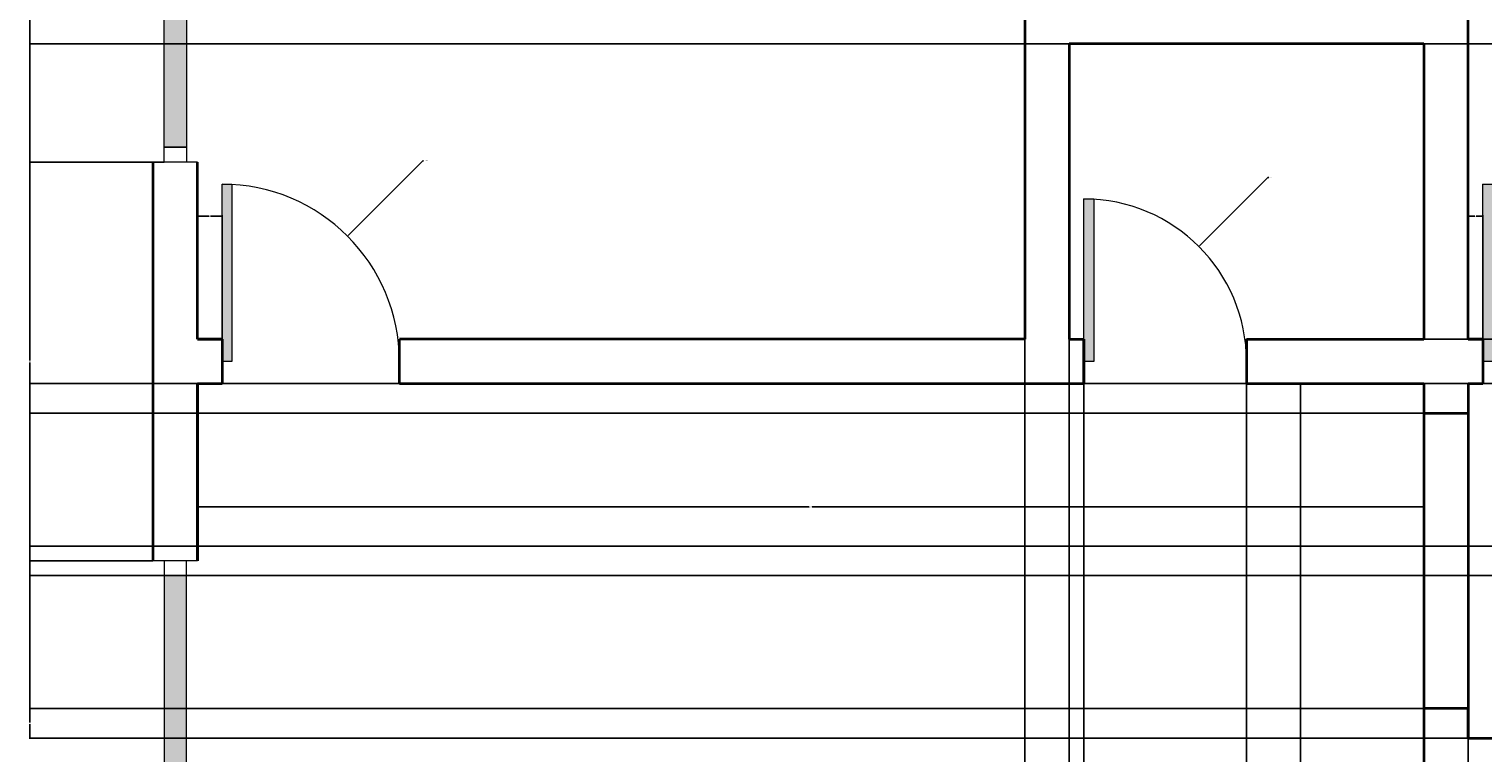
# Model space of a CAD drawing. Units: inches. Extents: x 2039 to 2485, y 1453 to 1986.
# Tile 2 of 4: x 2039 to 2334, y 1676 to 1823. Entities that reach past the tile are written whole.
import ezdxf

# ---------------------------------------------------------------- set-up
doc = ezdxf.new("R2010")
doc.units = ezdxf.units.IN
for name, color, linetype, lineweight in [('A-ANNO-DIMS', 2, 'Continuous', 18), ('A-DOOR', 3, 'Continuous', 18), ('A-GLAZ', 4, 'Continuous', 18), ('A-WALL', 7, 'Continuous', 35)]:
    doc.layers.add(name, color=color, linetype=linetype, lineweight=lineweight)
doc.layers.add('A-OPEN-PATT', color=18, linetype='Continuous', lineweight=13, true_color=0x000000)
doc.styles.get("Standard").update_dxf_attribs({"font": 'arial.ttf'})
doc.dimstyles.get("Standard").update_dxf_attribs({"dimtxt": 0.18, "dimasz": 0.18, "dimexe": 0.18, "dimexo": 0.0625, "dimgap": 0.09, "dimtad": 0, "dimtih": 1, "dimtoh": 1, "dimdec": 4, "dimzin": 0, "dimdsep": 46, "dimtxsty": 'Standard', "dimcen": 0.09, "dimadec": 0, "dimazin": 0, "dimtfac": 1, "dimtdec": 4, "dimtofl": 0, "dimtmove": 0, "dimatfit": 3, "dimfxl": 1, "dimtolj": 1, "dimtzin": 0, "dimarcsym": 0})

# ---------------------------------------------------------------- blocks, each defined once
blk = doc.blocks.new('DOOR-SWING-36IN')
for p, q in [((0, 0), (0, 36)), ((0, 36), (2, 36)), ((2, 36), (2, 0)), ((2, 0), (0, 0))]:
    blk.add_line(p, q)
blk.add_arc((0, 0), 36, 0, 90)
blk = doc.blocks.new('WIN-48IN')
for p, q in [((0, 48), (9, 48)), ((2.25, 3), (2.25, 48)), ((2.25, 48), (2.25, 45)), ((9, 48), (6.75, 48)), ((6.75, 48), (6.75, 0)), ((2.25, 45), (6.75, 45)), ((2.25, 0), (2.25, 3)), ((2.25, 3), (6.75, 3)), ((6.75, 3), (2.25, 3)), ((9, 0), (0, 0)), ((6.75, 0), (2.25, 0))]:
    blk.add_line(p, q)
blk = doc.blocks.new('*D27')
at = {"layer": 'A-ANNO-DIMS', "color": 0, "lineweight": -2, "transparency": 16777216}
for p, q in [((2063.94, 1796.06), (2038.81, 1796.06)), ((2038.99, 1795.88), (2038.99, 1755.74)), ((2038.99, 1715.24), (2038.99, 1755.37)), ((2063.94, 1715.06), (2038.81, 1715.06))]:
    blk.add_line(p, q, dxfattribs=at)
at = {"layer": 'A-ANNO-DIMS', "color": 0, "transparency": 16777216}
for points in [[(2038.96, 1795.88), (2039.02, 1795.88), (2038.99, 1796.06)], [(2038.96, 1715.24), (2039.02, 1715.24), (2038.99, 1715.06)]]:
    blk.add_solid(points, dxfattribs=at)
at = {"layer": 'Defpoints', "color": 0, "transparency": 16777216}
for p in [(2038.99, 1796.06), (2064, 1796.06), (2064, 1715.06)]:
    blk.add_point(p, dxfattribs=at)
at = {"layer": 'A-ANNO-DIMS', "color": 0, "transparency": 16777216, "insert": (2038.99, 1755.56), "char_height": 0.18, "attachment_point": 5}
blk.add_mtext('\\A1;81', dxfattribs=at)
blk = doc.blocks.new('*D28')
at = {"layer": 'A-ANNO-DIMS', "color": 0, "lineweight": -2, "transparency": 16777216}
for p, q in [((2063.94, 1856.06), (2038.81, 1856.06)), ((2038.99, 1855.88), (2038.99, 1826.24)), ((2038.99, 1796.24), (2038.99, 1825.87)), ((2063.94, 1796.06), (2038.81, 1796.06))]:
    blk.add_line(p, q, dxfattribs=at)
at = {"layer": 'A-ANNO-DIMS', "color": 0, "transparency": 16777216}
for points in [[(2038.96, 1855.88), (2039.02, 1855.88), (2038.99, 1856.06)], [(2038.96, 1796.24), (2039.02, 1796.24), (2038.99, 1796.06)]]:
    blk.add_solid(points, dxfattribs=at)
at = {"layer": 'Defpoints', "color": 0, "transparency": 16777216}
for p in [(2038.99, 1856.06), (2064, 1856.06), (2064, 1796.06)]:
    blk.add_point(p, dxfattribs=at)
at = {"layer": 'A-ANNO-DIMS', "color": 0, "transparency": 16777216, "insert": (2038.99, 1826.06), "char_height": 0.18, "attachment_point": 5}
blk.add_mtext('\\A1;60', dxfattribs=at)
blk = doc.blocks.new('*D34')
at = {"layer": 'A-ANNO-DIMS', "color": 0, "lineweight": -2, "transparency": 16777216}
for p, q in [((2073, 1760.12), (2073, 1785.25)), ((2073.18, 1785.07), (2075.35, 1785.07)), ((2077.82, 1785.07), (2075.65, 1785.07)), ((2078, 1760.12), (2078, 1785.25))]:
    blk.add_line(p, q, dxfattribs=at)
at = {"layer": 'A-ANNO-DIMS', "color": 0, "transparency": 16777216}
for points in [[(2073.18, 1785.1), (2073.18, 1785.04), (2073, 1785.07)], [(2077.82, 1785.1), (2077.82, 1785.04), (2078, 1785.07)]]:
    blk.add_solid(points, dxfattribs=at)
at = {"layer": 'Defpoints', "color": 0, "transparency": 16777216}
for p in [(2078, 1785.07), (2073, 1760.06), (2078, 1760.06)]:
    blk.add_point(p, dxfattribs=at)
at = {"layer": 'A-ANNO-DIMS', "color": 0, "transparency": 16777216, "insert": (2075.5, 1785.07), "char_height": 0.18, "attachment_point": 5}
blk.add_mtext('\\A1;5', dxfattribs=at)
blk = doc.blocks.new('*D35')
at = {"layer": 'A-ANNO-DIMS', "color": 0, "lineweight": -2, "transparency": 16777216}
for p, q in [((2331, 1760.12), (2331, 1785.25)), ((2331.18, 1785.07), (2332.35, 1785.07)), ((2333.82, 1785.07), (2332.65, 1785.07)), ((2334, 1760.12), (2334, 1785.25))]:
    blk.add_line(p, q, dxfattribs=at)
at = {"layer": 'A-ANNO-DIMS', "color": 0, "transparency": 16777216}
for points in [[(2331.18, 1785.1), (2331.18, 1785.04), (2331, 1785.07)], [(2333.82, 1785.1), (2333.82, 1785.04), (2334, 1785.07)]]:
    blk.add_solid(points, dxfattribs=at)
at = {"layer": 'Defpoints', "color": 0, "transparency": 16777216}
for p in [(2334, 1785.07), (2331, 1760.06), (2334, 1760.06)]:
    blk.add_point(p, dxfattribs=at)
at = {"layer": 'A-ANNO-DIMS', "color": 0, "transparency": 16777216, "insert": (2332.5, 1785.07), "char_height": 0.18, "attachment_point": 5}
blk.add_mtext('\\A1;3', dxfattribs=at)
blk = doc.blocks.new('*D39')
at = {"layer": 'A-ANNO-DIMS', "color": 0, "lineweight": -2, "transparency": 16777216}
for p, q in [((2073, 1750.99), (2073, 1725.87)), ((2322, 1750.99), (2322, 1725.87)), ((2073.18, 1726.05), (2197.21, 1726.05)), ((2321.82, 1726.05), (2197.79, 1726.05))]:
    blk.add_line(p, q, dxfattribs=at)
at = {"layer": 'A-ANNO-DIMS', "color": 0, "transparency": 16777216}
for points in [[(2073.18, 1726.08), (2073.18, 1726.02), (2073, 1726.05)], [(2321.82, 1726.08), (2321.82, 1726.02), (2322, 1726.05)]]:
    blk.add_solid(points, dxfattribs=at)
at = {"layer": 'Defpoints', "color": 0, "transparency": 16777216}
for p in [(2073, 1751.06), (2322, 1751.06), (2073, 1726.05)]:
    blk.add_point(p, dxfattribs=at)
at = {"layer": 'A-ANNO-DIMS', "color": 0, "transparency": 16777216, "insert": (2197.5, 1726.05), "char_height": 0.18, "attachment_point": 5}
blk.add_mtext('\\A1;249', dxfattribs=at)
blk = doc.blocks.new('*D40')
at = {"layer": 'A-ANNO-DIMS', "color": 0, "lineweight": -2, "transparency": 16777216}
for p, q in [((2321.94, 1751.06), (2296.81, 1751.06)), ((2296.99, 1750.88), (2296.99, 1619.24)), ((2296.99, 1487.24), (2296.99, 1618.87)), ((2321.94, 1487.06), (2296.81, 1487.06))]:
    blk.add_line(p, q, dxfattribs=at)
at = {"layer": 'A-ANNO-DIMS', "color": 0, "transparency": 16777216}
for points in [[(2296.96, 1750.88), (2297.02, 1750.88), (2296.99, 1751.06)], [(2296.96, 1487.24), (2297.02, 1487.24), (2296.99, 1487.06)]]:
    blk.add_solid(points, dxfattribs=at)
at = {"layer": 'Defpoints', "color": 0, "transparency": 16777216}
for p in [(2296.99, 1751.06), (2322, 1751.06), (2322, 1487.06)]:
    blk.add_point(p, dxfattribs=at)
at = {"layer": 'A-ANNO-DIMS', "color": 0, "transparency": 16777216, "insert": (2296.99, 1619.06), "char_height": 0.18, "attachment_point": 5}
blk.add_mtext('\\A1;264', dxfattribs=at)
blk = doc.blocks.new('*D42')
at = {"layer": 'A-ANNO-DIMS', "color": 0, "lineweight": -2, "transparency": 16777216}
for p, q in [((2241, 1759.99), (2241, 1452.87)), ((2250, 1759.99), (2250, 1452.87)), ((2241.18, 1453.05), (2245.35, 1453.05)), ((2249.82, 1453.05), (2245.65, 1453.05))]:
    blk.add_line(p, q, dxfattribs=at)
at = {"layer": 'A-ANNO-DIMS', "color": 0, "transparency": 16777216}
for points in [[(2241.18, 1453.08), (2241.18, 1453.02), (2241, 1453.05)], [(2249.82, 1453.08), (2249.82, 1453.02), (2250, 1453.05)]]:
    blk.add_solid(points, dxfattribs=at)
at = {"layer": 'Defpoints', "color": 0, "transparency": 16777216}
for p in [(2241, 1760.06), (2250, 1760.06), (2250, 1453.05)]:
    blk.add_point(p, dxfattribs=at)
at = {"layer": 'A-ANNO-DIMS', "color": 0, "transparency": 16777216, "insert": (2245.5, 1453.05), "char_height": 0.18, "attachment_point": 5}
blk.add_mtext('\\A1;9', dxfattribs=at)
blk = doc.blocks.new('*D48')
at = {"layer": 'A-ANNO-DIMS', "color": 0, "lineweight": -2, "transparency": 16777216}
for p, q in [((2322.06, 1820.06), (2485.19, 1820.06)), ((2485.01, 1819.88), (2485.01, 1790.24)), ((2485.01, 1760.24), (2485.01, 1789.87)), ((2322.06, 1760.06), (2485.19, 1760.06))]:
    blk.add_line(p, q, dxfattribs=at)
at = {"layer": 'A-ANNO-DIMS', "color": 0, "transparency": 16777216}
for points in [[(2484.98, 1819.88), (2485.04, 1819.88), (2485.01, 1820.06)], [(2484.98, 1760.24), (2485.04, 1760.24), (2485.01, 1760.06)]]:
    blk.add_solid(points, dxfattribs=at)
at = {"layer": 'Defpoints', "color": 0, "transparency": 16777216}
for p in [(2322, 1820.06), (2485.01, 1820.06), (2322, 1760.06)]:
    blk.add_point(p, dxfattribs=at)
at = {"layer": 'A-ANNO-DIMS', "color": 0, "transparency": 16777216, "insert": (2485.01, 1790.06), "char_height": 0.18, "attachment_point": 5}
blk.add_mtext('\\A1;60', dxfattribs=at)
blk = doc.blocks.new('*D49')
at = {"layer": 'A-ANNO-DIMS', "color": 0, "lineweight": -2, "transparency": 16777216}
for p, q in [((2249.94, 1826.06), (2038.81, 1826.06)), ((2038.99, 1825.88), (2038.99, 1823.24)), ((2038.99, 1820.24), (2038.99, 1822.87)), ((2249.94, 1820.06), (2038.81, 1820.06))]:
    blk.add_line(p, q, dxfattribs=at)
at = {"layer": 'A-ANNO-DIMS', "color": 0, "transparency": 16777216}
for points in [[(2038.96, 1825.88), (2039.02, 1825.88), (2038.99, 1826.06)], [(2038.96, 1820.24), (2039.02, 1820.24), (2038.99, 1820.06)]]:
    blk.add_solid(points, dxfattribs=at)
at = {"layer": 'Defpoints', "color": 0, "transparency": 16777216}
for p in [(2038.99, 1826.06), (2250, 1826.06), (2250, 1820.06)]:
    blk.add_point(p, dxfattribs=at)
at = {"layer": 'A-ANNO-DIMS', "color": 0, "transparency": 16777216, "insert": (2038.99, 1823.06), "char_height": 0.18, "attachment_point": 5}
blk.add_mtext('\\A1;6', dxfattribs=at)
blk = doc.blocks.new('*D54')
at = {"layer": 'A-ANNO-DIMS', "color": 0, "lineweight": -2, "transparency": 16777216}
for p, q in [((2250, 1759.99), (2250, 1452.87)), ((2253, 1750.99), (2253, 1452.87)), ((2250.18, 1453.05), (2251.35, 1453.05)), ((2252.82, 1453.05), (2251.65, 1453.05))]:
    blk.add_line(p, q, dxfattribs=at)
at = {"layer": 'A-ANNO-DIMS', "color": 0, "transparency": 16777216}
for points in [[(2250.18, 1453.08), (2250.18, 1453.02), (2250, 1453.05)], [(2252.82, 1453.08), (2252.82, 1453.02), (2253, 1453.05)]]:
    blk.add_solid(points, dxfattribs=at)
at = {"layer": 'Defpoints', "color": 0, "transparency": 16777216}
for p in [(2250, 1760.06), (2253, 1751.06), (2253, 1453.05)]:
    blk.add_point(p, dxfattribs=at)
at = {"layer": 'A-ANNO-DIMS', "color": 0, "transparency": 16777216, "insert": (2251.5, 1453.05), "char_height": 0.18, "attachment_point": 5}
blk.add_mtext('\\A1;3', dxfattribs=at)
blk = doc.blocks.new('*D55')
at = {"layer": 'A-ANNO-DIMS', "color": 0, "lineweight": -2, "transparency": 16777216}
for p, q in [((2253, 1750.99), (2253, 1452.87)), ((2286, 1750.99), (2286, 1452.87)), ((2253.18, 1453.05), (2269.28, 1453.05)), ((2285.82, 1453.05), (2269.72, 1453.05))]:
    blk.add_line(p, q, dxfattribs=at)
at = {"layer": 'A-ANNO-DIMS', "color": 0, "transparency": 16777216}
for points in [[(2253.18, 1453.08), (2253.18, 1453.02), (2253, 1453.05)], [(2285.82, 1453.08), (2285.82, 1453.02), (2286, 1453.05)]]:
    blk.add_solid(points, dxfattribs=at)
at = {"layer": 'Defpoints', "color": 0, "transparency": 16777216}
for p in [(2253, 1751.06), (2286, 1751.06), (2286, 1453.05)]:
    blk.add_point(p, dxfattribs=at)
at = {"layer": 'A-ANNO-DIMS', "color": 0, "transparency": 16777216, "insert": (2269.5, 1453.05), "char_height": 0.18, "attachment_point": 5}
blk.add_mtext('\\A1;33', dxfattribs=at)
blk = doc.blocks.new('*D56')
at = {"layer": 'A-ANNO-DIMS', "color": 0, "lineweight": -2, "transparency": 16777216}
for p, q in [((2286.06, 1760.06), (2485.19, 1760.06)), ((2485.01, 1759.88), (2485.01, 1755.74)), ((2485.01, 1751.24), (2485.01, 1755.37)), ((2286.06, 1751.06), (2485.19, 1751.06))]:
    blk.add_line(p, q, dxfattribs=at)
at = {"layer": 'A-ANNO-DIMS', "color": 0, "transparency": 16777216}
for points in [[(2484.98, 1759.88), (2485.04, 1759.88), (2485.01, 1760.06)], [(2484.98, 1751.24), (2485.04, 1751.24), (2485.01, 1751.06)]]:
    blk.add_solid(points, dxfattribs=at)
at = {"layer": 'Defpoints', "color": 0, "transparency": 16777216}
for p in [(2286, 1760.06), (2485.01, 1760.06), (2286, 1751.06)]:
    blk.add_point(p, dxfattribs=at)
at = {"layer": 'A-ANNO-DIMS', "color": 0, "transparency": 16777216, "insert": (2485.01, 1755.56), "char_height": 0.18, "attachment_point": 5}
blk.add_mtext('\\A1;9', dxfattribs=at)
blk = doc.blocks.new('*D58')
at = {"layer": 'A-ANNO-DIMS', "color": 0, "lineweight": -2, "transparency": 16777216}
for p, q in [((2331, 1678.99), (2331, 1452.87)), ((2352, 1678.99), (2352, 1452.87)), ((2331.18, 1453.05), (2341.3, 1453.05)), ((2351.82, 1453.05), (2341.71, 1453.05))]:
    blk.add_line(p, q, dxfattribs=at)
at = {"layer": 'A-ANNO-DIMS', "color": 0, "transparency": 16777216}
for points in [[(2331.18, 1453.08), (2331.18, 1453.02), (2331, 1453.05)], [(2351.82, 1453.08), (2351.82, 1453.02), (2352, 1453.05)]]:
    blk.add_solid(points, dxfattribs=at)
at = {"layer": 'Defpoints', "color": 0, "transparency": 16777216}
for p in [(2331, 1679.06), (2352, 1679.06), (2352, 1453.05)]:
    blk.add_point(p, dxfattribs=at)
at = {"layer": 'A-ANNO-DIMS', "color": 0, "transparency": 16777216, "insert": (2341.5, 1453.05), "char_height": 0.18, "attachment_point": 5}
blk.add_mtext('\\A1;21', dxfattribs=at)
blk = doc.blocks.new('*D61')
at = {"layer": 'A-ANNO-DIMS', "color": 0, "lineweight": -2, "transparency": 16777216}
for p, q in [((2351.94, 1751.06), (2038.81, 1751.06)), ((2038.99, 1750.88), (2038.99, 1734.74)), ((2038.99, 1718.24), (2038.99, 1734.37)), ((2351.94, 1718.06), (2038.81, 1718.06))]:
    blk.add_line(p, q, dxfattribs=at)
at = {"layer": 'A-ANNO-DIMS', "color": 0, "transparency": 16777216}
for points in [[(2038.96, 1750.88), (2039.02, 1750.88), (2038.99, 1751.06)], [(2038.96, 1718.24), (2039.02, 1718.24), (2038.99, 1718.06)]]:
    blk.add_solid(points, dxfattribs=at)
at = {"layer": 'Defpoints', "color": 0, "transparency": 16777216}
for p in [(2038.99, 1751.06), (2352, 1751.06), (2352, 1718.06)]:
    blk.add_point(p, dxfattribs=at)
at = {"layer": 'A-ANNO-DIMS', "color": 0, "transparency": 16777216, "insert": (2038.99, 1734.56), "char_height": 0.18, "attachment_point": 5}
blk.add_mtext('\\A1;33', dxfattribs=at)
blk = doc.blocks.new('*D62')
at = {"layer": 'A-ANNO-DIMS', "color": 0, "lineweight": -2, "transparency": 16777216}
for p, q in [((2351.94, 1718.06), (2038.81, 1718.06)), ((2038.99, 1717.88), (2038.99, 1715.24)), ((2038.99, 1712.24), (2038.99, 1714.87)), ((2351.94, 1712.06), (2038.81, 1712.06))]:
    blk.add_line(p, q, dxfattribs=at)
at = {"layer": 'A-ANNO-DIMS', "color": 0, "transparency": 16777216}
for points in [[(2038.96, 1717.88), (2039.02, 1717.88), (2038.99, 1718.06)], [(2038.96, 1712.24), (2039.02, 1712.24), (2038.99, 1712.06)]]:
    blk.add_solid(points, dxfattribs=at)
at = {"layer": 'Defpoints', "color": 0, "transparency": 16777216}
for p in [(2038.99, 1718.06), (2352, 1718.06), (2352, 1712.06)]:
    blk.add_point(p, dxfattribs=at)
at = {"layer": 'A-ANNO-DIMS', "color": 0, "transparency": 16777216, "insert": (2038.99, 1715.06), "char_height": 0.18, "attachment_point": 5}
blk.add_mtext('\\A1;6', dxfattribs=at)
blk = doc.blocks.new('*D63')
at = {"layer": 'A-ANNO-DIMS', "color": 0, "lineweight": -2, "transparency": 16777216}
for p, q in [((2321.94, 1745.06), (2038.81, 1745.06)), ((2038.99, 1744.88), (2038.99, 1715.24)), ((2038.99, 1685.24), (2038.99, 1714.87)), ((2321.94, 1685.06), (2038.81, 1685.06))]:
    blk.add_line(p, q, dxfattribs=at)
at = {"layer": 'A-ANNO-DIMS', "color": 0, "transparency": 16777216}
for points in [[(2038.96, 1744.88), (2039.02, 1744.88), (2038.99, 1745.06)], [(2038.96, 1685.24), (2039.02, 1685.24), (2038.99, 1685.06)]]:
    blk.add_solid(points, dxfattribs=at)
at = {"layer": 'Defpoints', "color": 0, "transparency": 16777216}
for p in [(2038.99, 1745.06), (2322, 1745.06), (2322, 1685.06)]:
    blk.add_point(p, dxfattribs=at)
at = {"layer": 'A-ANNO-DIMS', "color": 0, "transparency": 16777216, "insert": (2038.99, 1715.06), "char_height": 0.18, "attachment_point": 5}
blk.add_mtext('\\A1;60', dxfattribs=at)
blk = doc.blocks.new('*D64')
at = {"layer": 'A-ANNO-DIMS', "color": 0, "lineweight": -2, "transparency": 16777216}
for p, q in [((2330.94, 1685.06), (2038.81, 1685.06)), ((2038.99, 1684.88), (2038.99, 1682.24)), ((2038.99, 1679.24), (2038.99, 1681.87)), ((2330.94, 1679.06), (2038.81, 1679.06))]:
    blk.add_line(p, q, dxfattribs=at)
at = {"layer": 'A-ANNO-DIMS', "color": 0, "transparency": 16777216}
for points in [[(2038.96, 1684.88), (2039.02, 1684.88), (2038.99, 1685.06)], [(2038.96, 1679.24), (2039.02, 1679.24), (2038.99, 1679.06)]]:
    blk.add_solid(points, dxfattribs=at)
at = {"layer": 'Defpoints', "color": 0, "transparency": 16777216}
for p in [(2038.99, 1685.06), (2331, 1685.06), (2331, 1679.06)]:
    blk.add_point(p, dxfattribs=at)
at = {"layer": 'A-ANNO-DIMS', "color": 0, "transparency": 16777216, "insert": (2038.99, 1682.06), "char_height": 0.18, "attachment_point": 5}
blk.add_mtext('\\A1;6', dxfattribs=at)
blk = doc.blocks.new('*D66')
at = {"layer": 'A-ANNO-DIMS', "color": 0, "lineweight": -2, "transparency": 16777216}
for p, q in [((2118.73, 1796.29), (2103.59, 1781.14)), ((2118.91, 1796.29), (2118.73, 1796.29)), ((2077.91, 1755.56), (2078.09, 1755.56)), ((2078, 1755.47), (2078, 1755.65))]:
    blk.add_line(p, q, dxfattribs=at)
at = {"layer": 'A-ANNO-DIMS', "color": 0, "transparency": 16777216}
blk.add_solid([(2103.56, 1781.16), (2103.61, 1781.12), (2103.46, 1781.01)], dxfattribs=at)
at = {"layer": 'Defpoints', "color": 0, "transparency": 16777216}
for p in [(2103.46, 1781.01), (2078, 1755.56)]:
    blk.add_point(p, dxfattribs=at)
at = {"layer": 'A-ANNO-DIMS', "color": 0, "transparency": 16777216, "insert": (2119.41, 1796.29), "char_height": 0.18, "attachment_point": 5}
blk.add_mtext('\\A1;4X R36', dxfattribs=at)
blk = doc.blocks.new('*D67')
at = {"layer": 'A-ANNO-DIMS', "color": 0, "lineweight": -2, "transparency": 16777216}
for p, q in [((2290.34, 1792.89), (2276.46, 1779.02)), ((2290.52, 1792.89), (2290.34, 1792.89)), ((2252.91, 1755.56), (2253.09, 1755.56)), ((2253, 1755.47), (2253, 1755.65))]:
    blk.add_line(p, q, dxfattribs=at)
at = {"layer": 'A-ANNO-DIMS', "color": 0, "transparency": 16777216}
blk.add_solid([(2276.44, 1779.04), (2276.49, 1779), (2276.34, 1778.89)], dxfattribs=at)
at = {"layer": 'Defpoints', "color": 0, "transparency": 16777216}
for p in [(2276.34, 1778.89), (2253, 1755.56)]:
    blk.add_point(p, dxfattribs=at)
at = {"layer": 'A-ANNO-DIMS', "color": 0, "transparency": 16777216, "insert": (2290.82, 1792.89), "char_height": 0.18, "attachment_point": 5}
blk.add_mtext('\\A1;R33', dxfattribs=at)

msp = doc.modelspace()

# ---------------------------------------------------------------- hatches: boundary and pattern name
at = {"layer": 'A-OPEN-PATT'}
h = msp.add_hatch(color=256, dxfattribs=at)
h.dxf.hatch_style = 1
h.paths.add_polyline_path([(2070.75, 1853.06), (2066.25, 1853.06), (2066.25, 1799.06), (2070.75, 1799.06)])
h.paths.add_polyline_path([(2080, 1791.5, 0.013897), (2078, 1791.56), (2078, 1755.56), (2080, 1755.56)])
h.paths.add_polyline_path([(2070.75, 1712.06), (2066.25, 1712.06), (2066.25, 1670.06), (2070.75, 1670.06)])
h.paths.add_polyline_path([(2070.75, 1568.06), (2066.25, 1568.06), (2066.25, 1526.06), (2070.75, 1526.06)])
h.paths.add_polyline_path([(2080, 1518.5, 0.013897), (2078, 1518.56), (2078, 1482.56), (2080, 1482.56)])
h.paths.add_polyline_path([(2362.5, 1666.06), (2326.5, 1666.06), (2326.5, 1664.06), (2362.45, 1664.06, 0.013897)])
h.paths.add_polyline_path([(2457.75, 1601.06), (2453.25, 1601.06), (2453.25, 1553.06), (2457.75, 1553.06)])
h.paths.add_polyline_path([(2457.75, 1799.06), (2453.25, 1799.06), (2453.25, 1769.06), (2457.75, 1769.06)])
h.paths.add_polyline_path([(2336, 1791.5, 0.013897), (2334, 1791.56), (2334, 1755.56), (2336, 1755.56)])
h.paths.add_polyline_path([(2255, 1788.5, 0.015162), (2253, 1788.56), (2253, 1755.56), (2255, 1755.56)])
h.paths.add_polyline_path([(2331, 1830.06), (2322, 1830.06), (2322, 1828.06), (2331, 1828.06)])
h.paths.add_polyline_path([(2250, 1896.06), (2245.5, 1896.06), (2241, 1896.06), (2241, 1894.06), (2250, 1894.06)])
h.paths.add_polyline_path([(2271.5, 1896.06), (2250, 1896.06), (2250, 1894.06), (2271.5, 1894.06)])
h.paths.add_polyline_path([(2304, 1958.81), (2268, 1958.81), (2268, 1954.31), (2304, 1954.31)])

# ---------------------------------------------------------------- linework, layer by layer
at = {"layer": 'A-DOOR'}
for p, q in [((2253, 1755.56), (2253, 1788.56)), ((2253, 1788.56), (2255, 1788.56)), ((2255, 1788.56), (2255, 1755.56)), ((2255, 1755.56), (2253, 1755.56))]:
    msp.add_line(p, q, dxfattribs=at)
msp.add_arc((2253, 1755.56), 33, 360, 90, dxfattribs=at)
at = {"layer": 'A-GLAZ'}
for p, q in [((2066.25, 1799.06), (2066.25, 1856.06)), ((2070.75, 1856.06), (2070.75, 1796.06)), ((2066.25, 1796.06), (2066.25, 1799.06)), ((2066.25, 1799.06), (2070.75, 1799.06)), ((2070.75, 1799.06), (2066.25, 1799.06)), ((2073, 1796.06), (2064, 1796.06)), ((2070.75, 1796.06), (2064, 1796.06)), ((2064, 1796.06), (2066.25, 1796.06))]:
    msp.add_line(p, q, dxfattribs=at)
at = {"layer": 'A-WALL'}
for p, q in [((2241, 1896.06), (2241, 1760.06)), ((2331, 1760.06), (2331, 1830.06)), ((2322, 1820.06), (2250, 1820.06)), ((2250, 1820.06), (2250, 1760.06)), ((2322, 1820.06), (2322, 1760.06)), ((2064, 1715.06), (2064, 1796.06)), ((2073, 1760.06), (2073, 1796.06)), ((2073, 1760.06), (2073, 1796.06)), ((2073, 1760.06), (2078, 1760.06)), ((2078, 1760.06), (2073, 1760.06)), ((2078, 1760.06), (2078, 1751.06)), ((2241, 1760.06), (2114, 1760.06)), ((2114, 1751.06), (2114, 1760.06)), ((2250, 1760.06), (2253, 1760.06)), ((2250, 1760.06), (2253, 1760.06)), ((2253, 1760.06), (2253, 1751.06)), ((2253, 1751.06), (2253, 1760.06)), ((2286, 1760.06), (2286, 1751.06)), ((2286, 1760.06), (2322, 1760.06)), ((2331, 1760.06), (2334, 1760.06)), ((2334, 1760.06), (2331, 1760.06)), ((2334, 1760.06), (2334, 1751.06)), ((2073, 1751.06), (2078, 1751.06)), ((2073, 1751.06), (2078, 1751.06)), ((2073, 1751.06), (2073, 1715.06)), ((2073, 1715.06), (2073, 1751.06)), ((2114, 1751.06), (2253, 1751.06)), ((2114, 1751.06), (2253, 1751.06)), ((2286, 1751.06), (2322, 1751.06)), ((2286, 1751.06), (2322, 1751.06)), ((2322, 1751.06), (2322, 1666.06)), ((2322, 1751.06), (2322, 1745.06)), ((2331, 1751.06), (2334, 1751.06)), ((2331, 1751.06), (2331, 1679.06)), ((2322, 1745.06), (2331, 1745.06)), ((2331, 1685.06), (2322, 1685.06)), ((2331, 1679.06), (2331, 1685.06)), ((2331, 1679.06), (2451, 1679.06))]:
    msp.add_line(p, q, dxfattribs=at)

# ---------------------------------------------------------------- block references
at = {"layer": 'A-DOOR'}
for p in [(2078, 1755.56), (2334, 1755.56)]:
    msp.add_blockref('DOOR-SWING-36IN', p, dxfattribs=at)
at = {"layer": 'A-GLAZ', "extrusion": (0, 0, -1), "zscale": -1, "rotation": 180}
msp.add_blockref('WIN-48IN', (-2064, 1715.06), dxfattribs=at)

# ---------------------------------------------------------------- dimensions: what is measured, and where the dimension line sits
at = {"layer": 'A-ANNO-DIMS'}
for base, p1, p2, angle, picture, middle in [((2038.99, 1856.06), (2064, 1796.06), (2064, 1856.06), 90, '*D28', (2038.99, 1826.06)), ((2038.99, 1826.06), (2250, 1820.06), (2250, 1826.06), 90, '*D49', (2038.99, 1823.06)), ((2485.01, 1820.06), (2322, 1760.06), (2322, 1820.06), 90, '*D48', (2485.01, 1790.06)), ((2038.99, 1796.06), (2064, 1715.06), (2064, 1796.06), 90, '*D27', (2038.99, 1755.56)), ((2485.01, 1760.06), (2286, 1751.06), (2286, 1760.06), 90, '*D56', (2485.01, 1755.56)), ((2038.99, 1751.06), (2352, 1718.06), (2352, 1751.06), 90, '*D61', (2038.99, 1734.56)), ((2073, 1726.05), (2322, 1751.06), (2073, 1751.06), 180, '*D39', (2197.5, 1726.05)), ((2296.99, 1751.06), (2322, 1487.06), (2322, 1751.06), 90, '*D40', (2296.99, 1619.06)), ((2038.99, 1745.06), (2322, 1685.06), (2322, 1745.06), 90, '*D63', (2038.99, 1715.06)), ((2038.99, 1718.06), (2352, 1712.06), (2352, 1718.06), 90, '*D62', (2038.99, 1715.06)), ((2038.99, 1685.06), (2331, 1679.06), (2331, 1685.06), 90, '*D64', (2038.99, 1682.06))]:
    dim = msp.add_linear_dim(base=base, p1=p1, p2=p2, angle=angle, dimstyle='Standard', override={"dimdec": 0, "dimlfac": 1, "dimrnd": 0, "dimzin": 0, "dimdsep": 46, "dimlunit": 2}, dxfattribs=at)
    dim.commit()
    dim.dimension.update_dxf_attribs({"geometry": picture, "text_midpoint": middle})
dim = msp.add_radius_dim(center=(2078, 1755.56), mpoint=(2103.46, 1781.01), text='4X <>', dimstyle='Standard', override={"dimdec": 0, "dimlfac": 1, "dimrnd": 0, "dimzin": 0, "dimdsep": 46, "dimlunit": 2}, dxfattribs=at)
dim.commit()
dim.dimension.update_dxf_attribs({"geometry": '*D66', "text_midpoint": (2119.41, 1796.29), "dimtype": 164})
dim = msp.add_radius_dim(center=(2253, 1755.56), mpoint=(2276.34, 1778.89), dimstyle='Standard', override={"dimdec": 0, "dimlfac": 1, "dimrnd": 0, "dimzin": 0, "dimdsep": 46, "dimlunit": 2}, dxfattribs=at)
dim.commit()
dim.dimension.update_dxf_attribs({"geometry": '*D67', "text_midpoint": (2290.82, 1792.89), "dimtype": 164})
for base, p1, p2, picture, middle in [((2078, 1785.07), (2073, 1760.06), (2078, 1760.06), '*D34', (2075.5, 1785.07)), ((2334, 1785.07), (2331, 1760.06), (2334, 1760.06), '*D35', (2332.5, 1785.07)), ((2250, 1453.05), (2241, 1760.06), (2250, 1760.06), '*D42', (2245.5, 1453.05)), ((2253, 1453.05), (2250, 1760.06), (2253, 1751.06), '*D54', (2251.5, 1453.05)), ((2286, 1453.05), (2253, 1751.06), (2286, 1751.06), '*D55', (2269.5, 1453.05)), ((2352, 1453.05), (2331, 1679.06), (2352, 1679.06), '*D58', (2341.5, 1453.05))]:
    dim = msp.add_linear_dim(base=base, p1=p1, p2=p2, dimstyle='Standard', override={"dimdec": 0, "dimlfac": 1, "dimrnd": 0, "dimzin": 0, "dimdsep": 46, "dimlunit": 2}, dxfattribs=at)
    dim.commit()
    dim.dimension.update_dxf_attribs({"geometry": picture, "text_midpoint": middle})

doc.saveas('drawing.dxf')
